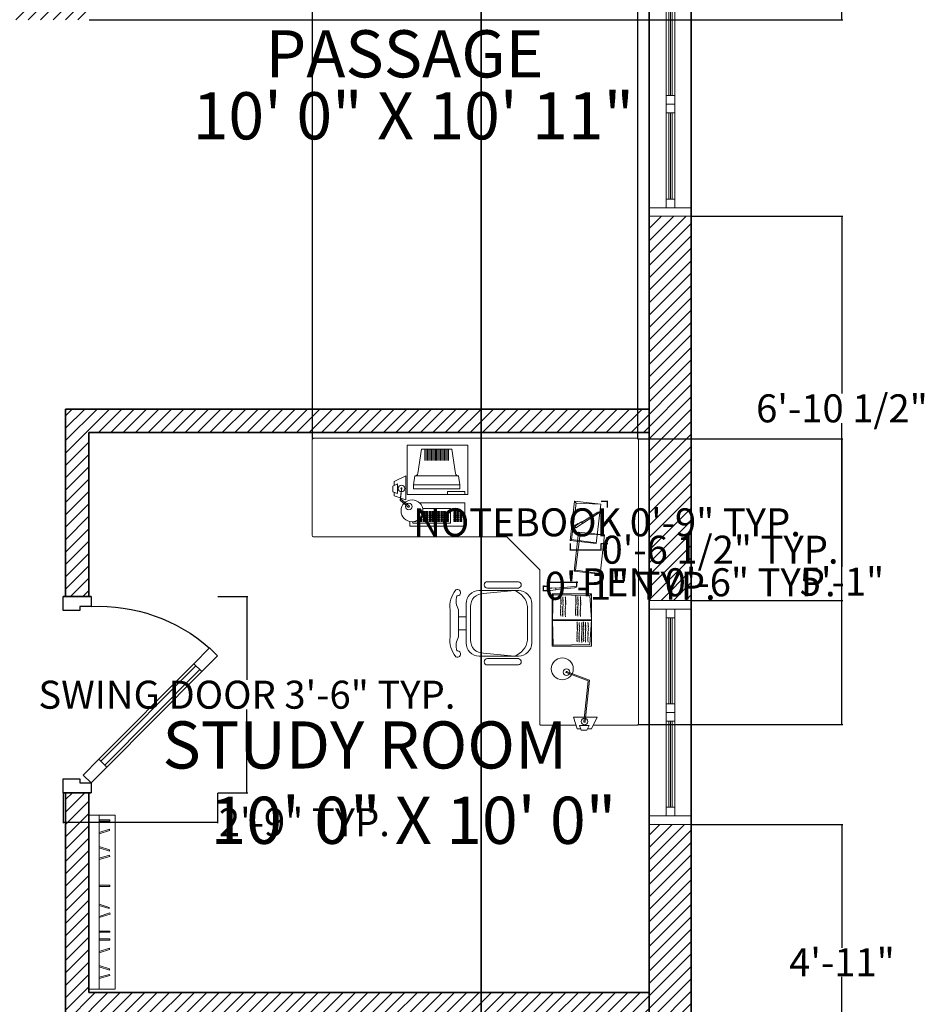
# Model space of a CAD drawing. Units: inches. Extents: x 585 to 1401, y -184 to 463.
# Tile 4 of 8: x 798 to 991, y 53 to 264. Entities that reach past the tile are written whole.
import ezdxf

# ---------------------------------------------------------------- set-up
doc = ezdxf.new("R2010")
doc.units = ezdxf.units.IN
doc.header["$MEASUREMENT"] = 0
for name, color, linetype, lineweight in [('A-ANNO-DIMS', 2, 'Continuous', 18), ('A-AREA-IDEN', 7, 'Continuous', 18), ('A-Door', 150, 'Continuous', 25), ('A-EQPM', 8, 'Continuous', 13), ('A-EQPM-PATT', 8, 'Continuous', 13), ('A-FURN', 8, 'Continuous', 18), ('A-Glaz', 140, 'Continuous', 18), ('A-Wall', 7, 'Continuous', 35), ('A-WALL-PATT', 252, 'Continuous', 13)]:
    doc.layers.add(name, color=color, linetype=linetype, lineweight=lineweight)
doc.styles.get("Standard").update_dxf_attribs({"font": 'arial.ttf'})
doc.dimstyles.get("Standard").update_dxf_attribs({"dimtxt": 6, "dimasz": 0.18, "dimexe": 0.18, "dimexo": 0.0625, "dimgap": 0.09, "dimtad": 0, "dimtih": 1, "dimtoh": 1, "dimdec": 0, "dimzin": 0, "dimdsep": 46, "dimlunit": 3, "dimtxsty": 'Standard', "dimblk": 'ARCHTICK', "dimcen": 0.09, "dimadec": 0, "dimazin": 0, "dimtfac": 1, "dimtdec": 0, "dimtofl": 0, "dimtmove": 0, "dimatfit": 3, "dimfxl": 1, "dimtolj": 1, "dimtzin": 0, "dimarcsym": 0})

# ---------------------------------------------------------------- blocks, each defined once
blk = doc.blocks.new('A$C1DF4181C')
blk.add_lwpolyline([(120, 128), (460.7, 466.1), (432.5, 494.5), (91.8, 156.4)], close=True)
blk.add_arc((72.4, 128.7), 593.3, 357.2313, 41.4937)
at = {"layer": 'A-Door'}
for points in [[(517.5, 522.4), (460.7, 466.1), (432.5, 494.5), (489.3, 550.8)], [(63.2, 71.6), (120, 128), (91.8, 156.4), (35, 100)], [(35, 100), (0, 100), (0, 0), (50, 0), (50, 50), (50, 60), (35, 60)], [(665, 100), (665, 60), (650, 60), (650, 50), (650, 0), (700, 0), (700, 100)]]:
    blk.add_lwpolyline(points, close=True, dxfattribs=at)
at = {"layer": 'A-Glaz'}
blk.add_lwpolyline([(112.9, 135.1), (453.6, 473.2), (439.5, 487.4), (98.8, 149.3)], close=True, dxfattribs=at)
at = {"layer": 'A-Wall'}
for p, q in [((0, 0), (0, 100)), ((0, 100), (0, 0)), ((700, 0), (700, 100)), ((700, 0), (700, 100))]:
    blk.add_line(p, q, dxfattribs=at)
blk = doc.blocks.new('WIN-48-DOUBLE-PANEL')
for p, q in [((48, 9), (0, 9)), ((0, 9), (0, 0)), ((1.85, 9), (0, 9)), ((0, 9), (0, 0)), ((1.85, 0), (1.85, 9)), ((1.85, 0), (1.85, 9)), ((46.15, 9), (48, 9)), ((46.15, 0), (46.15, 9)), ((46.15, 0), (46.15, 9)), ((46.15, 0), (46.15, 9)), ((48, 9), (48, 0)), ((48, 0), (48, 9)), ((1.85, 5.44), (46.15, 5.44)), ((3.69, 3.6), (3.69, 5.44)), ((3.69, 4.89), (22.15, 4.89)), ((3.69, 4.52), (22.15, 4.52)), ((22.15, 5.44), (22.15, 3.6)), ((24, 5.44), (24, 3.6)), ((25.85, 5.44), (25.85, 3.6)), ((44.31, 4.89), (25.85, 4.89)), ((44.31, 4.52), (25.85, 4.52)), ((44.31, 3.6), (44.31, 5.44)), ((1.85, 3.6), (46.15, 3.6)), ((3.69, 4.15), (22.15, 4.15)), ((44.31, 4.15), (25.85, 4.15)), ((0, 0), (1.85, 0)), ((48, 0), (0, 0)), ((48, 0), (46.15, 0))]:
    blk.add_line(p, q)
blk = doc.blocks.new('DESK-PEN')
for p, q in [((0, 0.46), (1.68, 0.61)), ((0.04, 0), (0, 0.46)), ((0.04, 0.56), (0.86, 0.63)), ((0.05, 0.44), (0.04, 0.56)), ((1.72, 0.15), (0.04, 0)), ((0.05, 0.44), (0.87, 0.51)), ((0.87, 0.51), (0.86, 0.63)), ((1.68, 0.61), (1.71, 0.23)), ((1.69, 0.51), (5.7, 0.87)), ((1.71, 0.23), (5.73, 0.59)), ((1.71, 0.23), (1.72, 0.15)), ((6.23, 0.79), (5.7, 0.87)), ((5.73, 0.59), (6.23, 0.79))]:
    blk.add_line(p, q)
blk = doc.blocks.new('DESK-NOTEBOOK')
for p, q in [((0.28, 0.83), (1.27, 8.63)), ((0.95, 9.02), (1.27, 8.63)), ((1.27, 8.63), (6.54, 8.39)), ((0.28, 0.83), (0, 0.63)), ((0.28, 0.83), (5.49, 0.12)), ((5.49, 0.12), (5.59, 0.01))]:
    blk.add_line(p, q)
blk.add_lwpolyline([(5.59, 0), (0, 0.63), (0.95, 9.02), (6.54, 8.39)], close=True)
blk = doc.blocks.new('_ArchTick')
at = {"color": 0, "linetype": 'ByBlock', "const_width": 0.15}
blk.add_lwpolyline([(-0.5, -0.5), (0.5, 0.5)], dxfattribs=at)
blk = doc.blocks.new('*D42')
at = {"layer": 'A-ANNO-DIMS', "color": 0, "lineweight": -2, "transparency": 16777216}
for p, q in [((840.14, 140.58), (846.56, 140.58)), ((846.38, 140.58), (846.38, 122.78)), ((846.38, 98.58), (846.38, 116.38)), ((840.14, 98.58), (846.56, 98.58))]:
    blk.add_line(p, q, dxfattribs=at)
at = {"layer": 'Defpoints', "color": 0, "transparency": 16777216}
for p in [(840.08, 140.58), (846.38, 140.58), (840.08, 98.58)]:
    blk.add_point(p, dxfattribs=at)
at = {"layer": 'A-ANNO-DIMS', "color": 0, "lineweight": -2, "transparency": 16777216, "xscale": 0.18, "yscale": 0.18, "zscale": 0.18}
for p, rotation in [((846.38, 140.58), 90), ((846.38, 98.58), 270)]:
    blk.add_blockref('_ArchTick', p, dxfattribs=dict(at, rotation=rotation))
at = {"layer": 'A-ANNO-DIMS', "color": 0, "transparency": 16777216, "insert": (846.38, 119.58), "char_height": 6, "attachment_point": 5}
blk.add_mtext('\\A1;SWING DOOR 3\'-6" TYP.', dxfattribs=at)
blk = doc.blocks.new('*D43')
at = {"layer": 'A-ANNO-DIMS', "color": 0, "lineweight": -2, "transparency": 16777216}
for p, q in [((807.03, 98.52), (807.03, 92.1)), ((840.08, 98.52), (840.08, 92.1)), ((807.03, 92.28), (840.08, 92.28)), ((840.08, 92.28), (840.26, 92.28))]:
    blk.add_line(p, q, dxfattribs=at)
at = {"layer": 'Defpoints', "color": 0, "transparency": 16777216}
for p in [(807.03, 98.58), (840.08, 98.58), (840.08, 92.28)]:
    blk.add_point(p, dxfattribs=at)
at = {"layer": 'A-ANNO-DIMS', "color": 0, "lineweight": -2, "transparency": 16777216, "xscale": 0.18, "yscale": 0.18, "zscale": 0.18, "rotation": 180}
blk.add_blockref('_ArchTick', (807.03, 92.28), dxfattribs=at)
at = {"layer": 'A-ANNO-DIMS', "color": 0, "lineweight": -2, "transparency": 16777216, "xscale": 0.18, "yscale": 0.18, "zscale": 0.18}
blk.add_blockref('_ArchTick', (840.08, 92.28), dxfattribs=at)
at = {"layer": 'A-ANNO-DIMS', "color": 0, "transparency": 16777216, "insert": (858.68, 92.28), "char_height": 6, "attachment_point": 5}
blk.add_mtext('\\A1;2\'-9" TYP.', dxfattribs=at)
blk = doc.blocks.new('*D72')
at = {"layer": 'A-ANNO-DIMS', "color": 0, "lineweight": -2, "transparency": 16777216}
for p, q in [((910.82, 142.79), (910.82, 143.84)), ((910.82, 143.66), (917.05, 143.66)), ((917.05, 142.79), (917.05, 143.84)), ((917.05, 143.66), (917.23, 143.66))]:
    blk.add_line(p, q, dxfattribs=at)
at = {"layer": 'Defpoints', "color": 0, "transparency": 16777216}
for p in [(917.05, 143.66), (910.82, 142.73), (917.05, 142.73)]:
    blk.add_point(p, dxfattribs=at)
at = {"layer": 'A-ANNO-DIMS', "color": 0, "lineweight": -2, "transparency": 16777216, "xscale": 0.18, "yscale": 0.18, "zscale": 0.18, "rotation": 180}
blk.add_blockref('_ArchTick', (910.82, 143.66), dxfattribs=at)
at = {"layer": 'A-ANNO-DIMS', "color": 0, "lineweight": -2, "transparency": 16777216, "xscale": 0.18, "yscale": 0.18, "zscale": 0.18}
blk.add_blockref('_ArchTick', (917.05, 143.66), dxfattribs=at)
at = {"layer": 'A-ANNO-DIMS', "color": 0, "transparency": 16777216, "insert": (945.24, 143.66), "char_height": 6, "attachment_point": 5}
blk.add_mtext('\\A1;PEN 0\'-6" TYP.', dxfattribs=at)
blk = doc.blocks.new('*D73')
at = {"layer": 'A-ANNO-DIMS', "color": 0, "lineweight": -2, "transparency": 16777216}
for p, q in [((910.76, 142.73), (909.71, 142.73)), ((910.76, 141.86), (909.71, 141.86)), ((909.89, 142.73), (909.89, 142.91)), ((909.89, 142.91), (910.07, 142.91)), ((909.89, 141.86), (909.89, 142.73))]:
    blk.add_line(p, q, dxfattribs=at)
at = {"layer": 'Defpoints', "color": 0, "transparency": 16777216}
for p in [(909.89, 142.73), (910.82, 142.73), (910.82, 141.86)]:
    blk.add_point(p, dxfattribs=at)
at = {"layer": 'A-ANNO-DIMS', "color": 0, "lineweight": -2, "transparency": 16777216, "xscale": 0.18, "yscale": 0.18, "zscale": 0.18}
for p, rotation in [((909.89, 142.73), 90), ((909.89, 141.86), 270)]:
    blk.add_blockref('_ArchTick', p, dxfattribs=dict(at, rotation=rotation))
at = {"layer": 'A-ANNO-DIMS', "color": 0, "transparency": 16777216, "insert": (928.44, 142.91), "char_height": 6, "attachment_point": 5}
blk.add_mtext('\\A1;0\'-1" TYP.', dxfattribs=at)
blk = doc.blocks.new('*D74')
at = {"layer": 'A-ANNO-DIMS', "color": 0, "lineweight": -2, "transparency": 16777216}
for p, q in [((922.2, 161.01), (923.67, 161.01)), ((923.49, 161.01), (923.49, 159.7)), ((922.2, 151.99), (923.67, 151.99)), ((923.49, 151.99), (923.49, 153.31))]:
    blk.add_line(p, q, dxfattribs=at)
at = {"layer": 'Defpoints', "color": 0, "transparency": 16777216}
for p in [(922.14, 161.01), (923.49, 161.01), (922.14, 151.99)]:
    blk.add_point(p, dxfattribs=at)
at = {"layer": 'A-ANNO-DIMS', "color": 0, "lineweight": -2, "transparency": 16777216, "xscale": 0.18, "yscale": 0.18, "zscale": 0.18}
for p, rotation in [((923.49, 161.01), 90), ((923.49, 151.99), 270)]:
    blk.add_blockref('_ArchTick', p, dxfattribs=dict(at, rotation=rotation))
at = {"layer": 'A-ANNO-DIMS', "color": 0, "transparency": 16777216, "insert": (923.49, 156.5), "char_height": 6, "attachment_point": 5}
blk.add_mtext('\\A1;NOTEBOOK 0\'-9" TYP.', dxfattribs=at)
blk = doc.blocks.new('*D75')
at = {"layer": 'A-ANNO-DIMS', "color": 0, "lineweight": -2, "transparency": 16777216}
for p, q in [((915.6, 151.93), (915.6, 150.46)), ((922.14, 151.93), (922.14, 150.46)), ((915.6, 150.64), (922.14, 150.64)), ((922.14, 150.64), (922.32, 150.64))]:
    blk.add_line(p, q, dxfattribs=at)
at = {"layer": 'Defpoints', "color": 0, "transparency": 16777216}
for p in [(915.6, 151.99), (922.14, 151.99), (922.14, 150.64)]:
    blk.add_point(p, dxfattribs=at)
at = {"layer": 'A-ANNO-DIMS', "color": 0, "lineweight": -2, "transparency": 16777216, "xscale": 0.18, "yscale": 0.18, "zscale": 0.18, "rotation": 180}
blk.add_blockref('_ArchTick', (915.6, 150.64), dxfattribs=at)
at = {"layer": 'A-ANNO-DIMS', "color": 0, "lineweight": -2, "transparency": 16777216, "xscale": 0.18, "yscale": 0.18, "zscale": 0.18}
blk.add_blockref('_ArchTick', (922.14, 150.64), dxfattribs=at)
at = {"layer": 'A-ANNO-DIMS', "color": 0, "transparency": 16777216, "insert": (947.68, 150.64), "char_height": 6, "attachment_point": 5}
blk.add_mtext('\\A1;0\'-6 1/2" TYP.', dxfattribs=at)
blk = doc.blocks.new('*D76')
at = {"layer": 'A-ANNO-DIMS', "color": 0, "lineweight": -2, "transparency": 16777216}
for p, q in [((654.47, 422.15), (622.1, 422.15)), ((622.28, 422.15), (622.28, 142.65)), ((622.28, -143.23), (622.28, 136.27)), ((807.47, -143.23), (622.1, -143.23))]:
    blk.add_line(p, q, dxfattribs=at)
at = {"layer": 'Defpoints', "color": 0, "transparency": 16777216}
for p in [(622.28, 422.15), (654.53, 422.15), (807.53, -143.23)]:
    blk.add_point(p, dxfattribs=at)
at = {"layer": 'A-ANNO-DIMS', "color": 0, "lineweight": -2, "transparency": 16777216, "xscale": 0.18, "yscale": 0.18, "zscale": 0.18}
for p, rotation in [((622.28, 422.15), 90), ((622.28, -143.23), 270)]:
    blk.add_blockref('_ArchTick', p, dxfattribs=dict(at, rotation=rotation))
at = {"layer": 'A-ANNO-DIMS', "color": 0, "transparency": 16777216, "insert": (622.28, 139.46), "char_height": 6, "attachment_point": 5}
blk.add_mtext('\\A1;47\'-1 1/2"', dxfattribs=at)
blk = doc.blocks.new('*D78')
at = {"layer": 'A-ANNO-DIMS', "color": 0, "lineweight": -2, "transparency": 16777216}
for p, q in [((860.46, 174.47), (860.46, 454.58)), ((860.46, 454.4), (880.22, 454.4)), ((930.1, 454.4), (910.34, 454.4)), ((930.1, 174.47), (930.1, 454.58))]:
    blk.add_line(p, q, dxfattribs=at)
at = {"layer": 'Defpoints', "color": 0, "transparency": 16777216}
for p in [(930.1, 454.4), (860.46, 174.41), (930.1, 174.41)]:
    blk.add_point(p, dxfattribs=at)
at = {"layer": 'A-ANNO-DIMS', "color": 0, "lineweight": -2, "transparency": 16777216, "xscale": 0.18, "yscale": 0.18, "zscale": 0.18, "rotation": 180}
blk.add_blockref('_ArchTick', (860.46, 454.4), dxfattribs=at)
at = {"layer": 'A-ANNO-DIMS', "color": 0, "lineweight": -2, "transparency": 16777216, "xscale": 0.18, "yscale": 0.18, "zscale": 0.18}
blk.add_blockref('_ArchTick', (930.1, 454.4), dxfattribs=at)
at = {"layer": 'A-ANNO-DIMS', "color": 0, "transparency": 16777216, "insert": (895.28, 454.4), "char_height": 6, "attachment_point": 5}
blk.add_mtext('\\A1;5\'-9 1/2"', dxfattribs=at)
blk = doc.blocks.new('*D79')
at = {"layer": 'A-ANNO-DIMS', "color": 0, "lineweight": -2, "transparency": 16777216}
for p, q in [((930.17, 174.41), (973.96, 174.41)), ((973.78, 174.41), (973.78, 146.95)), ((973.78, 113.18), (973.78, 140.64)), ((930.2, 113.18), (973.96, 113.18))]:
    blk.add_line(p, q, dxfattribs=at)
at = {"layer": 'Defpoints', "color": 0, "transparency": 16777216}
for p in [(930.1, 174.41), (930.14, 113.18), (973.78, 113.18)]:
    blk.add_point(p, dxfattribs=at)
at = {"layer": 'A-ANNO-DIMS', "color": 0, "lineweight": -2, "transparency": 16777216, "xscale": 0.18, "yscale": 0.18, "zscale": 0.18}
for p, rotation in [((973.78, 174.41), 90), ((973.78, 113.18), 270)]:
    blk.add_blockref('_ArchTick', p, dxfattribs=dict(at, rotation=rotation))
at = {"layer": 'A-ANNO-DIMS', "color": 0, "transparency": 16777216, "insert": (973.78, 143.8), "char_height": 6, "attachment_point": 5}
blk.add_mtext('\\A1;5\'-1"', dxfattribs=at)
blk = doc.blocks.new('*D83')
at = {"layer": 'A-ANNO-DIMS', "color": 0, "lineweight": -2, "transparency": 16777216}
for p, q in [((896.53, 413.09), (896.53, -175.66)), ((932.53, 413.09), (932.53, -175.66)), ((896.53, -175.48), (906.47, -175.48)), ((932.53, -175.48), (922.59, -175.48))]:
    blk.add_line(p, q, dxfattribs=at)
at = {"layer": 'Defpoints', "color": 0, "transparency": 16777216}
for p in [(896.53, 413.15), (932.53, 413.15), (932.53, -175.48)]:
    blk.add_point(p, dxfattribs=at)
at = {"layer": 'A-ANNO-DIMS', "color": 0, "lineweight": -2, "transparency": 16777216, "xscale": 0.18, "yscale": 0.18, "zscale": 0.18, "rotation": 180}
blk.add_blockref('_ArchTick', (896.53, -175.48), dxfattribs=at)
at = {"layer": 'A-ANNO-DIMS', "color": 0, "lineweight": -2, "transparency": 16777216, "xscale": 0.18, "yscale": 0.18, "zscale": 0.18}
blk.add_blockref('_ArchTick', (932.53, -175.48), dxfattribs=at)
at = {"layer": 'A-ANNO-DIMS', "color": 0, "transparency": 16777216, "insert": (914.53, -175.48), "char_height": 6, "attachment_point": 5}
blk.add_mtext('\\A1;3\'-0"', dxfattribs=at)
blk = doc.blocks.new('*D85')
at = {"layer": 'A-ANNO-DIMS', "color": 0, "lineweight": -2, "transparency": 16777216}
for p, q in [((941.59, 222.04), (973.96, 222.04)), ((973.78, 222.04), (973.78, 184.1)), ((973.78, 139.77), (973.78, 177.72)), ((941.59, 139.77), (973.96, 139.77))]:
    blk.add_line(p, q, dxfattribs=at)
at = {"layer": 'Defpoints', "color": 0, "transparency": 16777216}
for p in [(941.53, 222.04), (973.78, 222.04), (941.53, 139.77)]:
    blk.add_point(p, dxfattribs=at)
at = {"layer": 'A-ANNO-DIMS', "color": 0, "lineweight": -2, "transparency": 16777216, "xscale": 0.18, "yscale": 0.18, "zscale": 0.18}
for p, rotation in [((973.78, 222.04), 90), ((973.78, 139.77), 270)]:
    blk.add_blockref('_ArchTick', p, dxfattribs=dict(at, rotation=rotation))
at = {"layer": 'A-ANNO-DIMS', "color": 0, "transparency": 16777216, "insert": (973.78, 180.91), "char_height": 6, "attachment_point": 5}
blk.add_mtext('\\A1;6\'-10 1/2"', dxfattribs=at)
blk = doc.blocks.new('*D86')
at = {"layer": 'A-ANNO-DIMS', "color": 0, "lineweight": -2, "transparency": 16777216}
for p, q in [((941.59, 91.77), (973.96, 91.77)), ((973.78, 91.77), (973.78, 65.37)), ((973.78, 32.77), (973.78, 59.17)), ((941.59, 32.77), (973.96, 32.77))]:
    blk.add_line(p, q, dxfattribs=at)
at = {"layer": 'Defpoints', "color": 0, "transparency": 16777216}
for p in [(941.53, 91.77), (973.78, 91.77), (941.53, 32.77)]:
    blk.add_point(p, dxfattribs=at)
at = {"layer": 'A-ANNO-DIMS', "color": 0, "lineweight": -2, "transparency": 16777216, "xscale": 0.18, "yscale": 0.18, "zscale": 0.18}
for p, rotation in [((973.78, 91.77), 90), ((973.78, 32.77), 270)]:
    blk.add_blockref('_ArchTick', p, dxfattribs=dict(at, rotation=rotation))
at = {"layer": 'A-ANNO-DIMS', "color": 0, "transparency": 16777216, "insert": (973.78, 62.27), "char_height": 6, "attachment_point": 5}
blk.add_mtext('\\A1;4\'-11"', dxfattribs=at)
blk = doc.blocks.new('*D88')
at = {"layer": 'A-ANNO-DIMS', "color": 0, "lineweight": -2, "transparency": 16777216}
for p, q in [((896.53, -134.17), (896.53, 454.58)), ((896.53, 454.4), (906.47, 454.4)), ((932.53, 454.4), (922.59, 454.4)), ((932.53, -134.17), (932.53, 454.58))]:
    blk.add_line(p, q, dxfattribs=at)
at = {"layer": 'Defpoints', "color": 0, "transparency": 16777216}
for p in [(932.53, 454.4), (896.53, -134.23), (932.53, -134.23)]:
    blk.add_point(p, dxfattribs=at)
at = {"layer": 'A-ANNO-DIMS', "color": 0, "lineweight": -2, "transparency": 16777216, "xscale": 0.18, "yscale": 0.18, "zscale": 0.18, "rotation": 180}
blk.add_blockref('_ArchTick', (896.53, 454.4), dxfattribs=at)
at = {"layer": 'A-ANNO-DIMS', "color": 0, "lineweight": -2, "transparency": 16777216, "xscale": 0.18, "yscale": 0.18, "zscale": 0.18}
blk.add_blockref('_ArchTick', (932.53, 454.4), dxfattribs=at)
at = {"layer": 'A-ANNO-DIMS', "color": 0, "transparency": 16777216, "insert": (914.53, 454.4), "char_height": 6, "attachment_point": 5}
blk.add_mtext('\\A1;3\'-0"', dxfattribs=at)
blk = doc.blocks.new('*D89')
at = {"layer": 'A-ANNO-DIMS', "color": 0, "lineweight": -2, "transparency": 16777216}
for p, q in [((812.59, 269.15), (973.96, 269.15)), ((973.78, 269.15), (973.78, 269.33)), ((973.78, 269.33), (973.96, 269.33)), ((973.78, 264.15), (973.78, 269.15)), ((812.59, 264.15), (973.96, 264.15))]:
    blk.add_line(p, q, dxfattribs=at)
at = {"layer": 'Defpoints', "color": 0, "transparency": 16777216}
for p in [(812.53, 269.15), (973.78, 269.15), (812.53, 264.15)]:
    blk.add_point(p, dxfattribs=at)
at = {"layer": 'A-ANNO-DIMS', "color": 0, "lineweight": -2, "transparency": 16777216, "xscale": 0.18, "yscale": 0.18, "zscale": 0.18}
for p, rotation in [((973.78, 269.15), 90), ((973.78, 264.15), 270)]:
    blk.add_blockref('_ArchTick', p, dxfattribs=dict(at, rotation=rotation))
at = {"layer": 'A-ANNO-DIMS', "color": 0, "transparency": 16777216, "insert": (982.02, 269.33), "char_height": 6, "attachment_point": 5}
blk.add_mtext('\\A1;0\'-5"', dxfattribs=at)

msp = doc.modelspace()

# ---------------------------------------------------------------- hatches: boundary and pattern name
at = {"layer": 'A-EQPM-PATT'}
h = msp.add_hatch(dxfattribs=at)
h.set_pattern_fill('ANSI31', color=256, scale=2.251286, angle=45, style=0)
h.paths.add_polyline_path([(884.4, 169.72), (889.61, 169.72), (889.61, 172.19), (884.4, 172.19)])
at = {"layer": 'A-WALL-PATT'}
h = msp.add_hatch(dxfattribs=at)
h.set_pattern_fill('ANSI31', color=256, scale=15)
h.set_pattern_definition([(45, (599.059, -1e-14), (-1.325825, 1.325825), [])])
h.paths.add_polyline_path([(711.53, 422.15), (654.53, 422.15), (654.53, -109.85), (680.03, -109.85), (680.03, -100.85), (663.53, -100.85), (663.53, 48.87), (759.53, 48.87), (759.53, 57.87), (663.53, 57.87), (663.53, 144.15), (663.53, 264.15), (812.53, 264.15), (812.53, 269.15), (663.53, 269.15), (663.53, 413.15), (711.53, 413.15)])
h.paths.add_polyline_path([(753.53, -100.85), (728.03, -100.85), (728.03, -109.85), (753.53, -109.85)], flags=17)
h.paths.add_polyline_path([(812.53, -71.54), (807.53, -71.54), (807.53, -100.85), (795.53, -100.85), (795.53, -109.85), (807.53, -109.85), (807.53, -143.23), (848.53, -143.23), (848.53, -134.23), (812.53, -134.23)])
h.paths.add_polyline_path([(941.53, 8.77), (932.53, 8.77), (932.53, -9.23), (812.53, -9.23), (812.53, 5.77), (807.53, 5.77), (807.53, -29.54), (812.53, -29.54), (812.53, -14.23), (932.53, -14.23), (932.53, -134.23), (896.53, -134.23), (896.53, -143.23), (941.53, -143.23)])
h.paths.add_polyline_path([(941.53, 91.77), (932.53, 91.77), (932.53, 55.77), (812.53, 55.77), (812.53, 98.58), (807.53, 98.58), (807.53, 35.77), (812.53, 35.77), (812.53, 50.77), (932.53, 50.77), (932.53, 32.77), (941.53, 32.77)])
h.paths.add_polyline_path([(941.53, 222.04), (932.53, 222.04), (932.53, 180.77), (807.53, 180.77), (807.53, 140.58), (812.53, 140.58), (812.53, 175.77), (932.53, 175.77), (932.53, 139.77), (941.53, 139.77)])
h.paths.add_polyline_path([(941.53, 422.15), (896.53, 422.15), (896.53, 413.15), (932.53, 413.15), (932.53, 317.15), (896.53, 317.15), (896.53, 312.15), (932.53, 312.15), (932.53, 270.04), (941.53, 270.04)])
h.paths.add_polyline_path([(848.53, 422.15), (759.53, 422.15), (759.53, 413.15), (807.53, 413.15), (807.53, 312.15), (848.53, 312.15), (848.53, 317.15), (812.53, 317.15), (812.53, 413.15), (848.53, 413.15)])

# ---------------------------------------------------------------- linework, layer by layer
at = {"layer": 'A-EQPM'}
for p, q in [((893.69, 173), (880.66, 173)), ((880.66, 173), (880.66, 162.45)), ((893.69, 162.45), (893.69, 173)), ((883.76, 172.19), (882.99, 166.96)), ((890.28, 172.19), (883.76, 172.19)), ((890.28, 172.19), (891.05, 166.96)), ((878.62, 164.72), (877.62, 164.23)), ((880.42, 166.45), (877.93, 165.24)), ((877.93, 164.38), (877.93, 165.24)), ((878.62, 162.68), (878.62, 164.72)), ((880.42, 161.35), (880.42, 166.45)), ((882.35, 166.45), (882.07, 164.55)), ((891.98, 164.55), (882.07, 164.55)), ((882.07, 164.55), (882.07, 163.67)), ((882.35, 166.45), (891.69, 166.45)), ((891.98, 164.55), (891.69, 166.45)), ((891.98, 163.67), (891.98, 164.55)), ((877.62, 163.01), (877.62, 164.23)), ((877.62, 163.01), (878.62, 162.68)), ((877.93, 162.17), (877.93, 162.91)), ((879.45, 163.6), (879.16, 161.25)), ((879.55, 163.86), (879.29, 161.5)), ((880.66, 162.45), (893.69, 162.45)), ((882.07, 163.67), (891.98, 163.67)), ((893.07, 163.07), (889.35, 163.07)), ((889.35, 163.07), (889.35, 162.45)), ((893.07, 162.45), (893.07, 163.07)), ((877.93, 162.17), (880.42, 161.35)), ((879.16, 161.25), (880.94, 159.78)), ((879.29, 161.5), (881.1, 160.01)), ((893.07, 160.67), (883.36, 160.67)), ((893.07, 155.7), (893.07, 160.67)), ((889.96, 159.43), (884.04, 159.43)), ((889.96, 156.32), (889.96, 159.43)), ((881.27, 156.67), (881.27, 155.7)), ((881.9, 156.63), (881.9, 156.32)), ((881.9, 156.32), (889.96, 156.32)), ((881.27, 155.7), (893.07, 155.7)), ((919.72, 122.69), (914.93, 124.49)), ((919.47, 122.55), (914.7, 124.33)), ((918.52, 113.79), (919.47, 122.55)), ((918.79, 113.89), (919.72, 122.69)), ((916.27, 114.76), (921.37, 114.76)), ((917.09, 112.26), (916.27, 114.76)), ((921.37, 114.76), (920.16, 112.26)), ((917.09, 112.26), (917.83, 112.26)), ((917.93, 111.96), (917.6, 112.96)), ((917.6, 112.96), (919.64, 112.96)), ((917.93, 111.96), (919.16, 111.96)), ((919.64, 112.96), (919.16, 111.96)), ((919.3, 112.26), (920.16, 112.26))]:
    msp.add_line(p, q, dxfattribs=at)
for points in [[(884.54, 158.6), (884.14, 158.6), (884.14, 158.82), (884.54, 158.82)], [(884.54, 158.2), (884.14, 158.2), (884.14, 158.42), (884.54, 158.42)], [(885.12, 158.6), (884.71, 158.6), (884.71, 158.82), (885.12, 158.82)], [(885.12, 158.2), (884.71, 158.2), (884.71, 158.42), (885.12, 158.42)], [(885.79, 158.6), (885.39, 158.6), (885.39, 158.82), (885.79, 158.82)], [(885.79, 158.2), (885.39, 158.2), (885.39, 158.42), (885.79, 158.42)], [(886.39, 158.6), (885.99, 158.6), (885.99, 158.82), (886.39, 158.82)], [(886.39, 158.2), (885.99, 158.2), (885.99, 158.42), (886.39, 158.42)], [(887.07, 158.6), (886.66, 158.6), (886.66, 158.82), (887.07, 158.82)], [(887.07, 158.2), (886.66, 158.2), (886.66, 158.42), (887.07, 158.42)], [(887.6, 158.6), (887.2, 158.6), (887.2, 158.82), (887.6, 158.82)], [(887.6, 158.2), (887.2, 158.2), (887.2, 158.42), (887.6, 158.42)], [(888.28, 158.6), (887.88, 158.6), (887.88, 158.82), (888.28, 158.82)], [(888.28, 158.2), (887.88, 158.2), (887.88, 158.42), (888.28, 158.42)], [(888.88, 158.6), (888.48, 158.6), (888.48, 158.82), (888.88, 158.82)], [(888.88, 158.2), (888.48, 158.2), (888.48, 158.42), (888.88, 158.42)], [(889.55, 158.6), (889.15, 158.6), (889.15, 158.82), (889.55, 158.82)], [(889.55, 158.2), (889.15, 158.2), (889.15, 158.42), (889.55, 158.42)], [(891.1, 158.6), (890.7, 158.6), (890.7, 158.82), (891.1, 158.82)], [(891.1, 158.2), (890.7, 158.2), (890.7, 158.42), (891.1, 158.42)], [(891.7, 158.6), (891.3, 158.6), (891.3, 158.82), (891.7, 158.82)], [(891.7, 158.2), (891.3, 158.2), (891.3, 158.42), (891.7, 158.42)], [(892.37, 158.6), (891.97, 158.6), (891.97, 158.82), (892.37, 158.82)], [(892.37, 158.2), (891.97, 158.2), (891.97, 158.42), (892.37, 158.42)], [(883.27, 156.67), (882.87, 156.67), (882.87, 156.89), (883.27, 156.89)], [(883.86, 157.05), (883.46, 157.05), (883.46, 157.27), (883.86, 157.27)], [(883.86, 156.67), (883.46, 156.67), (883.46, 156.89), (883.86, 156.89)], [(884.54, 157.81), (884.14, 157.81), (884.14, 158.04), (884.54, 158.04)], [(884.54, 157.45), (884.14, 157.45), (884.14, 157.67), (884.54, 157.67)], [(884.54, 157.05), (884.14, 157.05), (884.14, 157.27), (884.54, 157.27)], [(884.54, 156.67), (884.14, 156.67), (884.14, 156.89), (884.54, 156.89)], [(885.12, 157.81), (884.71, 157.81), (884.71, 158.04), (885.12, 158.04)], [(885.12, 157.45), (884.71, 157.45), (884.71, 157.67), (885.12, 157.67)], [(885.12, 157.05), (884.71, 157.05), (884.71, 157.27), (885.12, 157.27)], [(885.12, 156.67), (884.71, 156.67), (884.71, 156.89), (885.12, 156.89)], [(885.79, 157.81), (885.39, 157.81), (885.39, 158.04), (885.79, 158.04)], [(885.79, 157.45), (885.39, 157.45), (885.39, 157.67), (885.79, 157.67)], [(885.79, 157.05), (885.39, 157.05), (885.39, 157.27), (885.79, 157.27)], [(885.79, 156.67), (885.39, 156.67), (885.39, 156.89), (885.79, 156.89)], [(886.39, 157.81), (885.99, 157.81), (885.99, 158.04), (886.39, 158.04)], [(886.39, 157.45), (885.99, 157.45), (885.99, 157.67), (886.39, 157.67)], [(886.39, 157.05), (885.99, 157.05), (885.99, 157.27), (886.39, 157.27)], [(886.39, 156.67), (885.99, 156.67), (885.99, 156.89), (886.39, 156.89)], [(887.07, 157.81), (886.66, 157.81), (886.66, 158.04), (887.07, 158.04)], [(887.07, 157.45), (886.66, 157.45), (886.66, 157.67), (887.07, 157.67)], [(887.07, 157.05), (886.66, 157.05), (886.66, 157.27), (887.07, 157.27)], [(887.07, 156.67), (886.66, 156.67), (886.66, 156.89), (887.07, 156.89)], [(887.6, 157.81), (887.2, 157.81), (887.2, 158.04), (887.6, 158.04)], [(887.6, 157.45), (887.2, 157.45), (887.2, 157.67), (887.6, 157.67)], [(887.6, 157.05), (887.2, 157.05), (887.2, 157.27), (887.6, 157.27)], [(887.6, 156.67), (887.2, 156.67), (887.2, 156.89), (887.6, 156.89)], [(888.28, 157.81), (887.88, 157.81), (887.88, 158.04), (888.28, 158.04)], [(888.28, 157.45), (887.88, 157.45), (887.88, 157.67), (888.28, 157.67)], [(888.28, 157.05), (887.88, 157.05), (887.88, 157.27), (888.28, 157.27)], [(888.28, 156.67), (887.88, 156.67), (887.88, 156.89), (888.28, 156.89)], [(888.88, 157.81), (888.48, 157.81), (888.48, 158.04), (888.88, 158.04)], [(888.88, 157.45), (888.48, 157.45), (888.48, 157.67), (888.88, 157.67)], [(888.88, 157.05), (888.48, 157.05), (888.48, 157.27), (888.88, 157.27)], [(888.88, 156.67), (888.48, 156.67), (888.48, 156.89), (888.88, 156.89)], [(889.55, 157.81), (889.15, 157.81), (889.15, 158.04), (889.55, 158.04)], [(889.55, 157.45), (889.15, 157.45), (889.15, 157.67), (889.55, 157.67)], [(889.55, 157.05), (889.15, 157.05), (889.15, 157.27), (889.55, 157.27)], [(889.55, 156.67), (889.15, 156.67), (889.15, 156.89), (889.55, 156.89)], [(891.1, 157.81), (890.7, 157.81), (890.7, 158.04), (891.1, 158.04)], [(891.1, 157.45), (890.7, 157.45), (890.7, 157.67), (891.1, 157.67)], [(891.1, 157.05), (890.7, 157.05), (890.7, 157.27), (891.1, 157.27)], [(891.1, 156.67), (890.7, 156.67), (890.7, 156.89), (891.1, 156.89)], [(891.7, 157.81), (891.3, 157.81), (891.3, 158.04), (891.7, 158.04)], [(891.7, 157.45), (891.3, 157.45), (891.3, 157.67), (891.7, 157.67)], [(891.7, 157.05), (891.3, 157.05), (891.3, 157.27), (891.7, 157.27)], [(891.7, 156.67), (891.3, 156.67), (891.3, 156.89), (891.7, 156.89)], [(892.37, 157.81), (891.97, 157.81), (891.97, 158.04), (892.37, 158.04)], [(892.37, 157.45), (891.97, 157.45), (891.97, 157.67), (892.37, 157.67)], [(892.37, 157.05), (891.97, 157.05), (891.97, 157.27), (892.37, 157.27)], [(892.37, 156.67), (891.97, 156.67), (891.97, 156.89), (892.37, 156.89)]]:
    msp.add_lwpolyline(points, close=True, dxfattribs=at)
for points in [[(882.59, 156.79), (882.59, 156.67), (882.19, 156.67), (882.19, 156.67)], [(883.27, 157.2), (883.27, 157.05), (883.08, 157.05)], [(883.69, 157.67), (883.86, 157.67), (883.86, 157.45), (883.52, 157.45)], [(883.86, 157.98), (883.86, 157.81), (883.78, 157.81)]]:
    msp.add_lwpolyline(points, dxfattribs=at)
for centre, radius in [((879.5, 163.73), 0.709), ((881.73, 158.97), 2.35), ((881.04, 159.88), 0.709), ((913.9, 125.12), 2.35), ((914.8, 124.43), 0.709), ((918.65, 113.84), 0.709)]:
    msp.add_circle(centre, radius, dxfattribs=at)
for centre, radius, start, end in [((882.38, 167.07), 0.624, 267.252, 353.5662), ((891.66, 167.07), 0.624, 186.4338, 272.748), ((879.5, 163.73), 0.141, 69.7638, 249.7638), ((881.02, 159.89), 0.141, 235.0249, 55.0249), ((914.82, 124.41), 0.141, 34.9751, 214.9751), ((918.65, 113.84), 0.141, 200.2362, 20.2362)]:
    msp.add_arc(centre, radius, start, end, dxfattribs=at)
at = {"layer": 'A-FURN'}
for p, q in [((902.04, 153.38), (909.08, 146.35)), ((904.54, 143.79), (897.87, 143.79)), ((904.54, 142.43), (897.87, 142.43)), ((911.72, 141.22), (911.94, 140.96)), ((911.94, 140.96), (911.82, 135.7)), ((911.94, 140.96), (919.81, 140.85)), ((920.16, 141.22), (919.81, 140.85)), ((919.81, 140.85), (920.16, 135.59)), ((893.34, 136.28), (891.69, 136.28)), ((911.82, 135.7), (911.72, 135.59)), ((911.94, 130.22), (911.82, 135.48)), ((911.82, 135.48), (920.16, 135.48)), ((919.81, 130.32), (920.16, 135.59)), ((893.34, 133.46), (891.69, 133.46)), ((911.94, 130.22), (919.81, 130.32)), ((904.54, 127.3), (897.87, 127.3)), ((904.54, 125.95), (897.87, 125.95)), ((812.53, 93.77), (812.53, 56.48)), ((818.18, 93.77), (812.53, 93.77)), ((814.73, 56.48), (814.73, 93.77)), ((818.18, 56.48), (818.18, 93.77)), ((818.18, 56.48), (812.53, 56.48))]:
    msp.add_line(p, q, dxfattribs=at)
for points in [[(902.04, 153.38), (860.66, 153.38, -0.414214), (860.37, 153.66), (860.37, 174.21, -0.414214), (860.66, 174.49), (909.36, 174.49)], [(909.36, 174.49), (929.9, 174.49, -0.414214), (930.19, 174.21), (930.19, 113.34, -0.414214), (929.9, 113.06), (920.55, 113.06)], [(916.83, 113.06), (909.36, 113.06, -0.414214), (909.08, 113.34), (909.08, 146.35)], [(891.09, 142.03, 0.207066), (889.87, 137.75), (889.87, 134.87)], [(907.35, 134.87), (907.35, 139.09, 0.414214), (904.54, 141.9), (896.1, 141.9, 0.418376), (893.34, 139.09), (893.34, 134.87)], [(906.47, 134.87), (906.47, 138.46, 0.28028), (903.65, 141.9), (897.01, 141.27, 0.418376), (894.26, 138.46), (894.26, 134.87)], [(891.35, 140.75, 0.214578), (891.69, 137.76), (891.69, 134.87)], [(891.09, 127.71, -0.207066), (889.87, 131.99), (889.87, 134.87)], [(891.35, 128.99, -0.214578), (891.69, 131.98), (891.69, 134.87)], [(907.35, 134.87), (907.35, 130.65, -0.414214), (904.54, 127.83), (896.1, 127.83, -0.418376), (893.34, 130.65), (893.34, 134.87)], [(906.47, 134.87), (906.47, 131.28, -0.28028), (903.65, 127.83), (897.01, 128.46, -0.418376), (894.26, 131.28), (894.26, 134.87)]]:
    msp.add_lwpolyline(points, format="xyb", dxfattribs=at)
for points in [[(911.72, 135.59), (911.72, 141.22), (920.16, 141.22), (920.16, 135.59)], [(911.72, 135.59), (911.72, 129.96), (920.16, 129.96), (920.16, 135.59)]]:
    msp.add_lwpolyline(points, close=True, dxfattribs=at)
for points in [[(814.73, 92.76), (817.01, 92.76), (817.01, 92.51), (814.73, 92.51)], [(814.73, 89.8), (816.98, 90.51), (816.93, 90.76), (814.73, 90.05)], [(814.73, 87.06), (816.98, 86.34), (816.93, 86.1), (814.73, 86.8)], [(814.73, 84.58), (816.97, 85.19), (817.01, 84.94), (814.73, 84.32)], [(814.73, 78.78), (817.01, 78.78), (817.01, 78.53), (814.73, 78.53)], [(814.73, 74.71), (816.91, 74.01), (816.86, 73.77), (814.73, 74.45)], [(814.73, 71.83), (817.1, 72.59), (817.05, 72.83), (814.73, 72.09)], [(814.73, 68.95), (817.01, 68.95), (817.01, 68.7), (814.73, 68.7)], [(814.73, 67.27), (817.01, 67.27), (817.01, 67.02), (814.73, 67.02)], [(814.73, 64.3), (816.98, 65.02), (816.93, 65.26), (814.73, 64.56)], [(814.73, 61.56), (816.98, 60.85), (816.93, 60.6), (814.73, 61.3)], [(814.73, 59.09), (816.97, 59.69), (817.01, 59.45), (814.73, 58.83)]]:
    msp.add_lwpolyline(points, dxfattribs=at)
for centre, radius, start, end in [((897.87, 143.11), 0.678, 90, 270), ((904.42, 143.11), 0.688, 280.358, 79.4219), ((891.44, 141.43), 0.688, 262.4652, 120.1772), ((891.44, 128.3), 0.688, 239.8228, 97.5348), ((897.87, 126.63), 0.678, 90, 270), ((904.42, 126.63), 0.688, 280.5781, 79.642)]:
    msp.add_arc(centre, radius, start, end, dxfattribs=at)
for points in [[(913.6, 136.43), (913.59, 136.52), (913.59, 136.67), (913.49, 136.88), (913.61, 137.06), (913.48, 137.24), (913.63, 137.43), (913.4, 137.6), (913.69, 137.78), (913.42, 137.94), (913.71, 138.16), (913.45, 138.31), (913.65, 138.45), (913.43, 138.67), (913.83, 138.99), (913.51, 139.13), (913.8, 139.35), (913.43, 139.63), (913.73, 139.78), (913.55, 139.84), (913.67, 139.95), (913.54, 140.07), (913.65, 140.25), (913.53, 140.41), (913.66, 140.53), (913.49, 140.59), (913.58, 140.63), (913.57, 140.66), (913.57, 140.67)], [(914.03, 136.31), (914.03, 136.41), (914.03, 136.55), (913.93, 136.77), (914.05, 136.94), (913.92, 137.13), (914.07, 137.31), (913.84, 137.48), (914.13, 137.66), (913.86, 137.82), (914.15, 138.04), (913.89, 138.19), (914.09, 138.34), (913.87, 138.55), (914.27, 138.87), (913.95, 139.01), (914.23, 139.24), (913.87, 139.51), (914.17, 139.66), (913.99, 139.72), (914.11, 139.83), (913.98, 139.95), (914.09, 140.13), (913.96, 140.29), (914.1, 140.41), (913.93, 140.47), (914.02, 140.51), (914.01, 140.54), (914.01, 140.55)], [(914.59, 136.28), (914.59, 136.38), (914.58, 136.52), (914.49, 136.74), (914.6, 136.91), (914.47, 137.1), (914.63, 137.28), (914.39, 137.45), (914.68, 137.63), (914.41, 137.79), (914.7, 138.02), (914.44, 138.16), (914.65, 138.31), (914.42, 138.52), (914.82, 138.84), (914.5, 138.99), (914.79, 139.21), (914.42, 139.48), (914.73, 139.63), (914.54, 139.69), (914.67, 139.8), (914.54, 139.93), (914.64, 140.1), (914.52, 140.26), (914.65, 140.38), (914.48, 140.44), (914.57, 140.48), (914.56, 140.51), (914.56, 140.53)], [(916.81, 136.49), (916.81, 136.58), (916.8, 136.73), (916.71, 136.94), (916.82, 137.12), (916.69, 137.3), (916.85, 137.49), (916.61, 137.66), (916.9, 137.83), (916.64, 138), (916.92, 138.22), (916.66, 138.37), (916.87, 138.51), (916.64, 138.72), (917.04, 139.04), (916.73, 139.19), (917.01, 139.41), (916.65, 139.69), (916.95, 139.84), (916.76, 139.9), (916.89, 140), (916.76, 140.13), (916.86, 140.31), (916.74, 140.47), (916.88, 140.59), (916.71, 140.65), (916.79, 140.69), (916.79, 140.72), (916.78, 140.73)], [(917.25, 136.37), (917.25, 136.47), (917.24, 136.61), (917.15, 136.82), (917.26, 137), (917.13, 137.18), (917.29, 137.37), (917.05, 137.54), (917.34, 137.72), (917.07, 137.88), (917.36, 138.1), (917.1, 138.25), (917.31, 138.4), (917.08, 138.61), (917.48, 138.93), (917.16, 139.07), (917.45, 139.3), (917.08, 139.57), (917.39, 139.72), (917.2, 139.78), (917.33, 139.89), (917.2, 140.01), (917.3, 140.19), (917.18, 140.35), (917.31, 140.47), (917.14, 140.53), (917.23, 140.57), (917.22, 140.6), (917.22, 140.61)], [(917.81, 136.34), (917.8, 136.44), (917.8, 136.58), (917.7, 136.79), (917.82, 136.97), (917.69, 137.15), (917.84, 137.34), (917.61, 137.51), (917.9, 137.69), (917.63, 137.85), (917.92, 138.07), (917.66, 138.22), (917.86, 138.37), (917.64, 138.58), (918.04, 138.9), (917.72, 139.04), (918.01, 139.27), (917.64, 139.54), (917.94, 139.69), (917.76, 139.75), (917.88, 139.86), (917.75, 139.98), (917.86, 140.16), (917.74, 140.32), (917.87, 140.44), (917.7, 140.5), (917.79, 140.54), (917.78, 140.57), (917.78, 140.58)], [(917.1, 130.93), (917.1, 131.02), (917.1, 131.17), (917, 131.38), (917.11, 131.56), (916.99, 131.74), (917.14, 131.93), (916.91, 132.1), (917.2, 132.28), (916.93, 132.44), (917.22, 132.66), (916.96, 132.81), (917.16, 132.95), (916.94, 133.17), (917.34, 133.49), (917.02, 133.63), (917.3, 133.85), (916.94, 134.13), (917.24, 134.28), (917.06, 134.34), (917.18, 134.45), (917.05, 134.57), (917.16, 134.75), (917.03, 134.91), (917.17, 135.03), (917, 135.09), (917.09, 135.13), (917.08, 135.16), (917.08, 135.17)], [(917.54, 130.81), (917.54, 130.91), (917.53, 131.05), (917.44, 131.27), (917.55, 131.44), (917.42, 131.63), (917.58, 131.81), (917.34, 131.98), (917.64, 132.16), (917.37, 132.32), (917.65, 132.55), (917.4, 132.69), (917.6, 132.84), (917.37, 133.05), (917.78, 133.37), (917.46, 133.51), (917.74, 133.74), (917.38, 134.01), (917.68, 134.16), (917.5, 134.22), (917.62, 134.33), (917.49, 134.45), (917.6, 134.63), (917.47, 134.79), (917.61, 134.91), (917.44, 134.97), (917.52, 135.01), (917.52, 135.04), (917.51, 135.06)], [(918.1, 130.78), (918.09, 130.88), (918.09, 131.02), (917.99, 131.24), (918.11, 131.41), (917.98, 131.6), (918.13, 131.78), (917.9, 131.95), (918.19, 132.13), (917.92, 132.29), (918.21, 132.52), (917.95, 132.66), (918.15, 132.81), (917.93, 133.02), (918.33, 133.34), (918.01, 133.49), (918.3, 133.71), (917.93, 133.98), (918.24, 134.13), (918.05, 134.19), (918.18, 134.3), (918.05, 134.43), (918.15, 134.6), (918.03, 134.76), (918.16, 134.89), (917.99, 134.94), (918.08, 134.98), (918.07, 135.01), (918.07, 135.03)], [(918.45, 130.96), (918.45, 131.05), (918.44, 131.2), (918.34, 131.41), (918.46, 131.59), (918.33, 131.77), (918.49, 131.96), (918.25, 132.13), (918.54, 132.31), (918.27, 132.47), (918.56, 132.69), (918.3, 132.84), (918.51, 132.98), (918.28, 133.2), (918.68, 133.52), (918.36, 133.66), (918.65, 133.88), (918.28, 134.16), (918.59, 134.31), (918.4, 134.37), (918.53, 134.47), (918.4, 134.6), (918.5, 134.78), (918.38, 134.94), (918.51, 135.06), (918.34, 135.12), (918.43, 135.16), (918.42, 135.19), (918.42, 135.2)], [(918.89, 130.84), (918.88, 130.94), (918.88, 131.08), (918.78, 131.3), (918.9, 131.47), (918.77, 131.65), (918.92, 131.84), (918.69, 132.01), (918.98, 132.19), (918.71, 132.35), (919, 132.57), (918.74, 132.72), (918.94, 132.87), (918.72, 133.08), (919.12, 133.4), (918.8, 133.54), (919.09, 133.77), (918.72, 134.04), (919.03, 134.19), (918.84, 134.25), (918.96, 134.36), (918.83, 134.48), (918.94, 134.66), (918.82, 134.82), (918.95, 134.94), (918.78, 135), (918.87, 135.04), (918.86, 135.07), (918.86, 135.08)], [(919.44, 130.81), (919.44, 130.91), (919.43, 131.05), (919.34, 131.27), (919.45, 131.44), (919.32, 131.63), (919.48, 131.81), (919.25, 131.98), (919.54, 132.16), (919.27, 132.32), (919.55, 132.55), (919.3, 132.69), (919.5, 132.84), (919.27, 133.05), (919.68, 133.37), (919.36, 133.51), (919.64, 133.74), (919.28, 134.01), (919.58, 134.16), (919.4, 134.22), (919.52, 134.33), (919.39, 134.45), (919.5, 134.63), (919.37, 134.79), (919.51, 134.91), (919.34, 134.97), (919.42, 135.01), (919.42, 135.04), (919.41, 135.06)]]:
    msp.add_open_spline(points, degree=3, knots=[0, 0, 0, 0, 0.290305, 0.438765, 0.664768, 0.808263, 1.034266, 1.191713, 1.440843, 1.567995, 1.872124, 1.999284, 2.200678, 2.277764, 2.791434, 2.892138, 3.060765, 3.494351, 3.596167, 3.696867, 3.810729, 3.89123, 4.148149, 4.290596, 4.40446, 4.506274, 4.557181, 4.593196, 4.593196, 4.593196, 4.593196], dxfattribs=at)
at = {"layer": 'A-Wall'}
for p, q in [((941.53, 422.15), (941.53, -143.23)), ((932.53, 312.15), (932.53, 180.77)), ((807.53, 180.77), (932.53, 180.77)), ((807.53, 180.77), (807.53, 140.58)), ((812.53, 175.77), (932.53, 175.77)), ((812.53, 175.77), (812.53, 140.58)), ((932.53, 175.77), (932.53, 55.77)), ((812.53, 140.58), (807.53, 140.58)), ((812.53, 98.58), (807.53, 98.58)), ((807.53, 98.58), (807.53, 35.77)), ((812.53, 98.58), (812.53, 55.77)), ((812.53, 55.77), (932.53, 55.77))]:
    msp.add_line(p, q, dxfattribs=at)

# ---------------------------------------------------------------- block references
at = {"layer": 'A-Door', "xscale": -0.0599999999683043, "yscale": 0.0599999999683043, "zscale": 0.0599999999683043, "rotation": 270}
msp.add_blockref('A$C1DF4181C', (807.03, 98.58), dxfattribs=at)
at = {"layer": 'A-FURN'}
for name, p in [('DESK-NOTEBOOK', (915.6, 151.99)), ('DESK-NOTEBOOK', (916.43, 145.4)), ('DESK-PEN', (910.82, 141.86))]:
    msp.add_blockref(name, p, dxfattribs=at)
at = {"layer": 'A-FURN', "rotation": 27.07850367264702}
msp.add_blockref('DESK-PEN', (916.8, 155.3), dxfattribs=at)
at = {"layer": 'A-Glaz', "rotation": 270.0000000000021}
for p in [(932.53, 270.04), (932.53, 139.77)]:
    msp.add_blockref('WIN-48-DOUBLE-PANEL', p, dxfattribs=at)

# ---------------------------------------------------------------- texts
at = {"layer": 'A-AREA-IDEN'}
for s, height, p in [('PASSAGE', 10.101, (850.37, 251.79)), ('10\' 0" X 10\' 11"', 10.1013, (834.77, 238.52)), ('STUDY ROOM', 10.101, (828.3, 103.77)), ('10\' 0" X 10\' 0"', 10.1013, (838.59, 87.63))]:
    msp.add_text(s, height=height, dxfattribs=at).set_placement(p)

# ---------------------------------------------------------------- dimensions: what is measured, and where the dimension line sits
at = {"layer": 'A-ANNO-DIMS'}
for base, p1, p2, picture, middle in [((930.1, 454.4), (860.46, 174.41), (930.1, 174.41), '*D78', (895.28, 454.4)), ((932.53, 454.4), (896.53, -134.23), (932.53, -134.23), '*D88', (914.53, 454.4)), ((932.53, -175.48), (896.53, 413.15), (932.53, 413.15), '*D83', (914.53, -175.48))]:
    dim = msp.add_linear_dim(base=base, p1=p1, p2=p2, dimstyle='Standard', override={"dimdec": 1, "dimlfac": 1, "dimrnd": 0, "dimzin": 1, "dimdsep": 46, "dimlunit": 4, "dimfrac": 2}, dxfattribs=at)
    dim.commit()
    dim.dimension.update_dxf_attribs({"geometry": picture, "text_midpoint": middle})
for base, p1, p2, picture, middle in [((622.28, 422.15), (807.53, -143.23), (654.53, 422.15), '*D76', (622.28, 139.46)), ((973.78, 269.15), (812.53, 264.15), (812.53, 269.15), '*D89', (982.02, 269.33)), ((973.78, 222.04), (941.53, 139.77), (941.53, 222.04), '*D85', (973.78, 180.91)), ((973.78, 113.18), (930.1, 174.41), (930.14, 113.18), '*D79', (973.78, 143.8)), ((973.78, 91.77), (941.53, 32.77), (941.53, 91.77), '*D86', (973.78, 62.27))]:
    dim = msp.add_linear_dim(base=base, p1=p1, p2=p2, angle=90, dimstyle='Standard', override={"dimdec": 1, "dimlfac": 1, "dimrnd": 0, "dimzin": 1, "dimdsep": 46, "dimlunit": 4, "dimfrac": 2}, dxfattribs=at)
    dim.commit()
    dim.dimension.update_dxf_attribs({"geometry": picture, "text_midpoint": middle})
for base, p1, p2, text, picture, middle in [((923.49, 161.01), (922.14, 151.99), (922.14, 161.01), 'NOTEBOOK <> TYP.', '*D74', (923.49, 156.5)), ((909.89, 142.73), (910.82, 141.86), (910.82, 142.73), '<> TYP.', '*D73', (928.44, 142.91)), ((846.38, 140.58), (840.08, 98.58), (840.08, 140.58), 'SWING DOOR <> TYP.', '*D42', (846.38, 119.58))]:
    dim = msp.add_linear_dim(base=base, p1=p1, p2=p2, angle=90, text=text, dimstyle='Standard', override={"dimdec": 1, "dimlfac": 1, "dimrnd": 0, "dimzin": 1, "dimdsep": 46, "dimlunit": 4, "dimfrac": 2}, dxfattribs=at)
    dim.commit()
    dim.dimension.update_dxf_attribs({"geometry": picture, "text_midpoint": middle})
for base, p1, p2, text, picture, middle in [((922.14, 150.64), (915.6, 151.99), (922.14, 151.99), '<> TYP.', '*D75', (947.68, 150.64)), ((917.05, 143.66), (910.82, 142.73), (917.05, 142.73), 'PEN <> TYP.', '*D72', (945.24, 143.66)), ((840.0761, 92.2811), (807.0279, 98.5811), (840.0761, 98.5811), '<> TYP.', '*D43', (858.6838, 92.2811))]:
    dim = msp.add_linear_dim(base=base, p1=p1, p2=p2, text=text, dimstyle='Standard', override={"dimdec": 1, "dimlfac": 1, "dimrnd": 0, "dimzin": 1, "dimdsep": 46, "dimlunit": 4, "dimfrac": 2}, dxfattribs=at)
    dim.commit()
    dim.dimension.update_dxf_attribs({"geometry": picture, "text_midpoint": middle})

doc.saveas('drawing.dxf')
